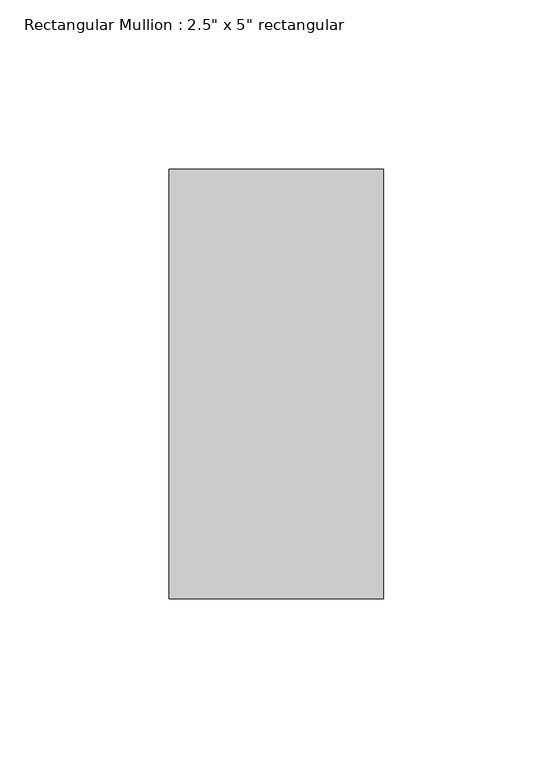
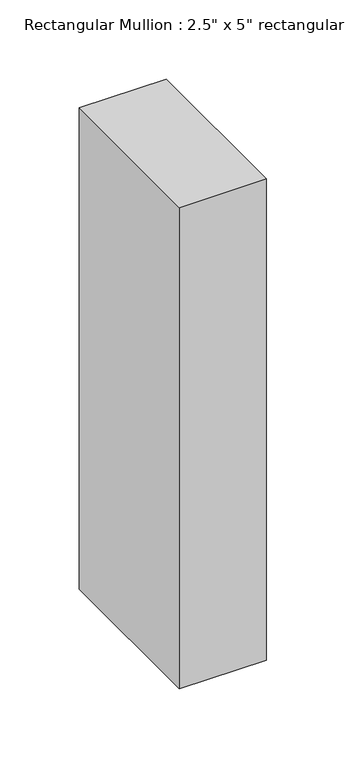
"""IFC4 building model written with IfcOpenShell, lengths in millimetres: member geometry."""

from ifc_helpers import new_model, si_unit, frame, origin, place, context, project, spatial, polyline, outline, extrude, source, transform, mapped, element, save


def member_f0218dda(model_context):
    return source(origin(), model_context, "Body", "SweptSolid", [
        extrude(outline(polyline([(0.0, 63.5), (0.0, -63.5), (-63.5, -63.5), (-63.5, 63.5), (0.0, 63.5)])), frame((0.0, 0.0, -371.5546147), z_axis=(0.0, 0.0, 1.0), x_axis=(1.0, 0.0, 0.0)), (0.0, 0.0, 1.0), 371.5546147),
    ])


if __name__ == "__main__":
    model = new_model("IFC4")
    model_context = context("Model", 3, world=origin())
    ifc_project = project(units=[si_unit("LENGTHUNIT", "METRE", prefix="MILLI")], contexts=[model_context])
    site = spatial("IfcSite", under=ifc_project)
    building = spatial("IfcBuilding", under=site)
    placement = place(None, origin())
    member_shape = member_f0218dda(model_context)
    element("IfcMember", 1, ObjectType="Rectangular Mullion : 2.5\" x 5\" rectangular", at=placement, inside=building, context=model_context, shape_type="MappedRepresentation", body=[
        mapped(member_shape, transform((0.0, 0.0, 0.0), x_axis=(1.0, 0.0, 0.0), y_axis=(0.0, 1.0, 0.0), z_axis=(0.0, 0.0, 1.0))),
    ])
    save(model, "model.ifc")

# Revit data of these elements
# Type "Rectangular Mullion : 2.5\" x 5\" rectangular"
#   built-in parameter 1007304 = 0.416667 (stored number, unit not read)
#   built-in parameter 1007301 = 0.104167 (stored number, unit not read)
#   built-in parameter 1007300 = 0.104167 (stored number, unit not read)
